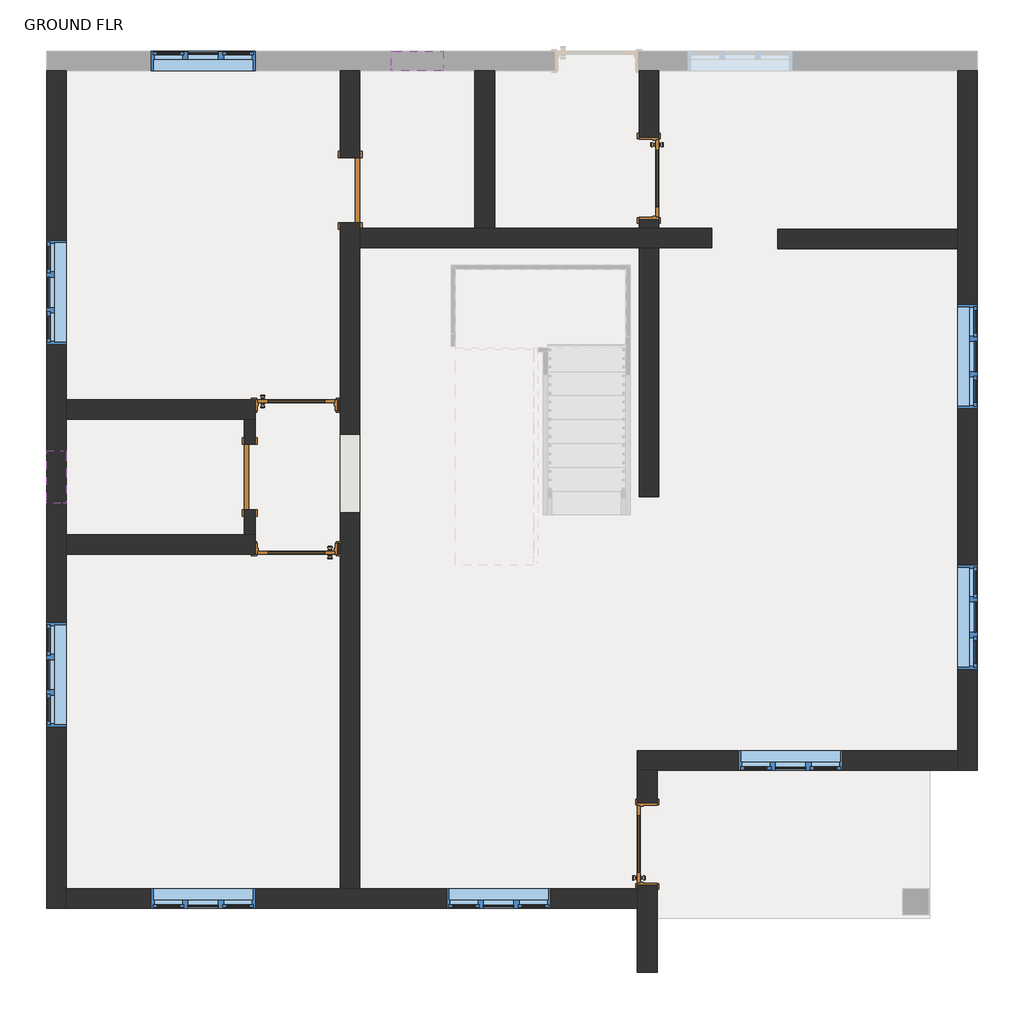
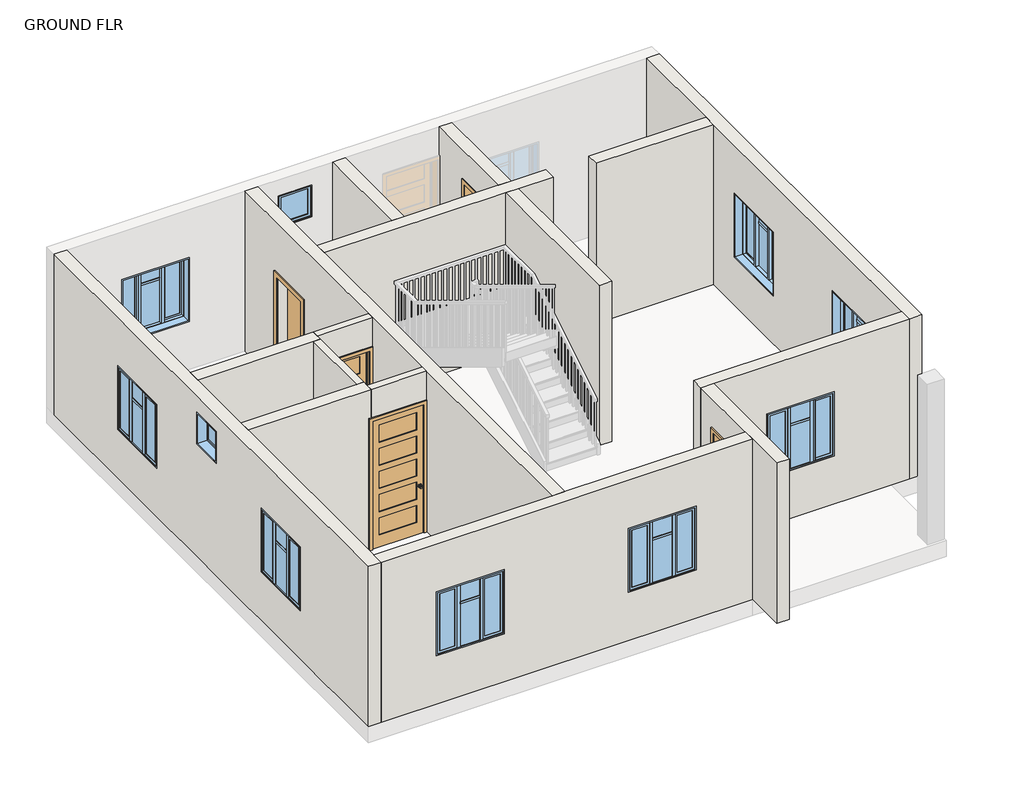
# One storey, part 1 of 3: 15 walls, 10 windows, 6 doors.
"""IFC4 building model written with IfcOpenShell, lengths in millimetres."""

from ifc_helpers import new_model, si_unit, point, frame, origin, place, context, project, spatial, polyline, ellipse_curve, trimmed, outline, extrude, faceted_brep, transform, mapped, element, save
from ifc_brep_helpers import plane_surface, extruded_surface, advanced_brep
from components import door_d793c26e, door_7b78131b, door_1fe7f57d, door_a1484949, window_80340324, window_casement_triple_middle_transom_window_4_x_4_1416bf83

model = new_model("IFC4")

# Units and contexts
model_context = context("Model", 3, world=origin())
ifc_project = project(units=[si_unit("LENGTHUNIT", "METRE", prefix="MILLI")], contexts=[model_context])

# Site, building, storey
site = spatial("IfcSite", under=ifc_project)
building = spatial("IfcBuilding", under=site)
storey = spatial("IfcBuildingStorey", under=building, Name="GROUND FLR", Elevation=609.6)

# Doors
placement = place(None, origin())
door_shape = door_d793c26e(model_context)
element("IfcDoor", 1, ObjectType="Door-Interior-Single-5_Panel_Vert-Wood : 36\" x 96\"", at=placement, inside=storey, context=model_context, shape_type="MappedRepresentation", body=[
    mapped(door_shape, transform((-5132.6956632, -7100.6948807, 609.6), x_axis=(0.0, 1.0, 0.0), y_axis=(-1.0, 0.0, 0.0), z_axis=(0.0, 0.0, 1.0))),
])
element("IfcDoor", 2, ObjectType="Door-Interior-Single-5_Panel_Vert-Wood : 36\" x 96\"", at=placement, inside=storey, context=model_context, shape_type="MappedRepresentation", body=[
    mapped(door_shape, transform((-5108.2681792, 684.4051193, 609.6), x_axis=(0.0, -1.0, 0.0), y_axis=(1.0, 0.0, 0.0), z_axis=(0.0, 0.0, 1.0))),
])
door_2_shape = door_7b78131b(model_context)
element("IfcDoor", 3, ObjectType="Door-Interior-Single-5_Panel_Vert-Wood : 36\" x 96\"", at=placement, inside=storey, context=model_context, shape_type="MappedRepresentation", body=[
    mapped(door_2_shape, transform((-9231.6206632, -3649.4698807, 609.6), x_axis=(-1.0, 0.0, 0.0), y_axis=(0.0, -1.0, 0.0), z_axis=(0.0, 0.0, 1.0))),
])
element("IfcDoor", 4, ObjectType="Door-Interior-Single-5_Panel_Vert-Wood : 36\" x 96\"", at=placement, inside=storey, context=model_context, shape_type="MappedRepresentation", body=[
    mapped(door_2_shape, transform((-9231.6206632, -1966.7198807, 609.6), x_axis=(1.0, 0.0, 0.0), y_axis=(0.0, 1.0, 0.0), z_axis=(0.0, 0.0, 1.0))),
])
door_3_shape = door_1fe7f57d(model_context)
element("IfcDoor", 5, ObjectType="Single-Flush : 30\" x 80\"", at=placement, inside=storey, context=model_context, shape_type="MappedRepresentation", body=[
    mapped(door_3_shape, transform((-9777.7206632, -2808.0948807, 609.6), x_axis=(0.0, 1.0, 0.0), y_axis=(-1.0, 0.0, 0.0), z_axis=(0.0, 0.0, 1.0))),
])
door_4_shape = door_a1484949(model_context)
element("IfcDoor", 6, ObjectType="Single-Flush : 30\" x 80\"", at=placement, inside=storey, context=model_context, shape_type="MappedRepresentation", body=[
    mapped(door_4_shape, transform((-8603.9431792, 544.7051193, 609.6), x_axis=(0.0, -1.0, 0.0), y_axis=(1.0, 0.0, 0.0), z_axis=(0.0, 0.0, 1.0))),
])

# Walls
element("IfcWall", 7, ObjectType="INTERIOR WALL 5\"", at=placement, inside=storey, context=model_context, shape_type="SweptSolid", body=[
    extrude(outline(polyline([(-2134.9948807, 609.6), (-2427.0948807, 609.6), (-2427.0948807, 2641.6), (-3189.0948807, 2641.6), (-3189.0948807, 609.6), (-3481.1948807, 609.6), (-3481.1948807, 3657.6), (-2134.9948807, 3657.6), (-2134.9948807, 609.6)])), frame((-9841.2206632, 0.0, 0.0), z_axis=(1.0, 0.0, 0.0), x_axis=(0.0, 1.0, 0.0)), (0.0, 0.0, 1.0), 127.0),
])
element("IfcWall", 8, ObjectType="INTERIOR WALL 5\"", at=placement, inside=storey, context=model_context, shape_type="SweptSolid", body=[
    extrude(outline(polyline([(3657.6, -8718.2431792), (3657.6, -9714.2206632), (3073.4, -9714.2206632), (3073.4, -8749.0206632), (609.6, -8749.0206632), (609.6, -8718.2431792), (3657.6, -8718.2431792)])), frame((0.0, -3709.7948807, 0.0), z_axis=(0.0, 1.0, 0.0), x_axis=(0.0, 0.0, 1.0)), (0.0, 0.0, 1.0), 127.0),
])
element("IfcWall", 9, ObjectType="INTERIOR WALL 5\"", at=placement, inside=storey, context=model_context, shape_type="SweptSolid", body=[
    extrude(outline(polyline([(3657.6, -8718.2431792), (3657.6, -9714.2206632), (3073.4, -9714.2206632), (3073.4, -8749.0206632), (609.6, -8749.0206632), (609.6, -8718.2431792), (3657.6, -8718.2431792)])), frame((0.0, -2033.3948807, 0.0), z_axis=(0.0, 1.0, 0.0), x_axis=(0.0, 0.0, 1.0)), (0.0, 0.0, 1.0), 127.0),
])
element("IfcWall", 10, ObjectType="WALL 9\"", at=placement, inside=storey, context=model_context, shape_type="Brep", body=[
    faceted_brep([(-12152.6206632, 1941.7051193, 609.6), (-12152.6206632, -7849.9948807, 609.6), (-12152.6206632, -7849.9948807, 3657.6), (-12152.6206632, 1941.7051193, 3657.6), (-12152.6206632, -39.4948807, 2743.2), (-12152.6206632, -1258.6948807, 2743.2), (-12152.6206632, -1258.6948807, 1524.0), (-12152.6206632, -39.4948807, 1524.0), (-12152.6206632, -4509.8948807, 2743.2), (-12152.6206632, -5729.0948807, 2743.2), (-12152.6206632, -5729.0948807, 1524.0), (-12152.6206632, -4509.8948807, 1524.0), (-12152.6206632, -3112.8948807, 3352.8), (-12152.6206632, -3112.8948807, 2743.2), (-12152.6206632, -2503.2948807, 2743.2), (-12152.6206632, -2503.2948807, 3352.8), (-11924.0206632, 1941.7051193, 609.6), (-11924.0206632, 1941.7051193, 3657.6), (-11924.0206632, -1906.3948807, 3657.6), (-11924.0206632, -2134.9948807, 3657.6), (-11924.0206632, -3481.1948807, 3657.6), (-11924.0206632, -3709.7948807, 3657.6), (-11924.0206632, -7621.3948807, 3657.6), (-11924.0206632, -7849.9948807, 3657.6), (-11924.0206632, -7849.9948807, 609.6), (-11924.0206632, -7621.3948807, 609.6), (-11924.0206632, -3709.7948807, 609.6), (-11924.0206632, -3481.1948807, 609.6), (-11924.0206632, -2134.9948807, 609.6), (-11924.0206632, -1906.3948807, 609.6), (-11924.0206632, -39.4948807, 2743.2), (-11924.0206632, -39.4948807, 1524.0), (-11924.0206632, -1258.6948807, 1524.0), (-11924.0206632, -1258.6948807, 2743.2), (-11924.0206632, -4509.8948807, 2743.2), (-11924.0206632, -4509.8948807, 1524.0), (-11924.0206632, -5729.0948807, 1524.0), (-11924.0206632, -5729.0948807, 2743.2), (-11924.0206632, -3112.8948807, 3352.8), (-11924.0206632, -2503.2948807, 3352.8), (-11924.0206632, -2503.2948807, 2743.2), (-11924.0206632, -3112.8948807, 2743.2)], [[[0, 1, 2, 3], [4, 5, 6, 7], [8, 9, 10, 11], [12, 13, 14, 15]], [[16, 17, 18, 19, 20, 21, 22, 23, 24, 25, 26, 27, 28, 29], [30, 31, 32, 33], [34, 35, 36, 37], [38, 39, 40, 41]], [[1, 0, 16, 29, 28, 27, 26, 25, 24]], [[3, 2, 23, 22, 21, 20, 19, 18, 17]], [[0, 3, 17, 16]], [[2, 1, 24, 23]], [[31, 30, 4, 7]], [[32, 31, 7, 6]], [[33, 32, 6, 5]], [[30, 33, 5, 4]], [[35, 34, 8, 11]], [[36, 35, 11, 10]], [[37, 36, 10, 9]], [[34, 37, 9, 8]], [[13, 12, 38, 41]], [[14, 13, 41, 40]], [[15, 14, 40, 39]], [[12, 15, 39, 38]]]),
])
element("IfcWall", 11, ObjectType="WALL 9\"", at=placement, inside=storey, context=model_context, shape_type="Brep", body=[
    faceted_brep([(-1497.3206632, 1941.7051193, 609.6), (-1497.3206632, 87.5051193, 609.6), (-1497.3206632, -141.0948807, 609.6), (-1497.3206632, -6008.4948807, 609.6), (-1497.3206632, -6237.0948807, 609.6), (-1497.3206632, -6237.0948807, 3657.6), (-1497.3206632, -6008.4948807, 3657.6), (-1497.3206632, -141.0948807, 3657.6), (-1497.3206632, 87.5051193, 3657.6), (-1497.3206632, 1941.7051193, 3657.6), (-1497.3206632, -5055.9948807, 2743.2), (-1497.3206632, -5055.9948807, 1524.0), (-1497.3206632, -3836.7948807, 1524.0), (-1497.3206632, -3836.7948807, 2743.2), (-1497.3206632, -2007.9948807, 2743.2), (-1497.3206632, -2007.9948807, 1524.0), (-1497.3206632, -788.7948807, 1524.0), (-1497.3206632, -788.7948807, 2743.2), (-1268.7206632, 1941.7051193, 609.6), (-1268.7206632, 1941.7051193, 3657.6), (-1268.7206632, -6237.0948807, 3657.6), (-1268.7206632, -6237.0948807, 609.6), (-1268.7206632, -5055.9948807, 2743.2), (-1268.7206632, -3836.7948807, 2743.2), (-1268.7206632, -3836.7948807, 1524.0), (-1268.7206632, -5055.9948807, 1524.0), (-1268.7206632, -2007.9948807, 2743.2), (-1268.7206632, -788.7948807, 2743.2), (-1268.7206632, -788.7948807, 1524.0), (-1268.7206632, -2007.9948807, 1524.0)], [[[0, 1, 2, 3, 4, 5, 6, 7, 8, 9], [10, 11, 12, 13], [14, 15, 16, 17]], [[18, 19, 20, 21], [22, 23, 24, 25], [26, 27, 28, 29]], [[4, 3, 2, 1, 0, 18, 21]], [[9, 8, 7, 6, 5, 20, 19]], [[0, 9, 19, 18]], [[5, 4, 21, 20]], [[11, 10, 22, 25]], [[12, 11, 25, 24]], [[13, 12, 24, 23]], [[10, 13, 23, 22]], [[15, 14, 26, 29]], [[16, 15, 29, 28]], [[17, 16, 28, 27]], [[14, 17, 27, 26]]]),
])
element("IfcWall", 12, ObjectType="WALL 9\"", at=placement, inside=storey, context=model_context, shape_type="SweptSolid", body=[
    extrude(outline(polyline([(-3605.5206632, 87.5051193), (-1497.3206632, 87.5051193), (-1497.3206632, -141.0948807), (-3605.5206632, -141.0948807), (-3605.5206632, 87.5051193)])), frame((0.0, 0.0, 609.6), z_axis=(0.0, 0.0, 1.0), x_axis=(1.0, 0.0, 0.0)), (0.0, 0.0, 1.0), 3048.0),
])
element("IfcWall", 13, ObjectType="WALL 9\"", at=placement, inside=storey, context=model_context, shape_type="Brep", body=[
    faceted_brep([(-11924.0206632, -7849.9948807, 609.6), (-5243.8206632, -7849.9948807, 609.6), (-5243.8206632, -7849.9948807, 3657.6), (-11924.0206632, -7849.9948807, 3657.6), (-10930.7319212, -7849.9948807, 2743.2), (-9711.5319212, -7849.9948807, 2743.2), (-9711.5319212, -7849.9948807, 1524.0), (-10930.7319212, -7849.9948807, 1524.0), (-7476.3319212, -7849.9948807, 2743.2), (-6257.1319212, -7849.9948807, 2743.2), (-6257.1319212, -7849.9948807, 1524.0), (-7476.3319212, -7849.9948807, 1524.0), (-11924.0206632, -7621.3948807, 609.6), (-11924.0206632, -7621.3948807, 3657.6), (-8718.2431792, -7621.3948807, 3657.6), (-8489.6431792, -7621.3948807, 3657.6), (-5243.8206632, -7621.3948807, 3657.6), (-5243.8206632, -7621.3948807, 609.6), (-8489.6431792, -7621.3948807, 609.6), (-8718.2431792, -7621.3948807, 609.6), (-10930.7319212, -7621.3948807, 2743.2), (-10930.7319212, -7621.3948807, 1524.0), (-9711.5319212, -7621.3948807, 1524.0), (-9711.5319212, -7621.3948807, 2743.2), (-7476.3319212, -7621.3948807, 2743.2), (-7476.3319212, -7621.3948807, 1524.0), (-6257.1319212, -7621.3948807, 1524.0), (-6257.1319212, -7621.3948807, 2743.2)], [[[0, 1, 2, 3], [4, 5, 6, 7], [8, 9, 10, 11]], [[12, 13, 14, 15, 16, 17, 18, 19], [20, 21, 22, 23], [24, 25, 26, 27]], [[1, 0, 12, 19, 18, 17]], [[3, 2, 16, 15, 14, 13]], [[0, 3, 13, 12]], [[2, 1, 17, 16]], [[21, 20, 4, 7]], [[22, 21, 7, 6]], [[23, 22, 6, 5]], [[20, 23, 5, 4]], [[25, 24, 8, 11]], [[26, 25, 11, 10]], [[27, 26, 10, 9]], [[24, 27, 9, 8]]]),
])
element("IfcWall", 14, ObjectType="WALL 9\"", at=placement, inside=storey, context=model_context, shape_type="Brep", body=[
    faceted_brep([(-5015.2206632, -6237.0948807, 3657.6), (-5015.2206632, -8599.2948807, 3657.6), (-5015.2206632, -8599.2948807, 609.6), (-5015.2206632, -7583.2948807, 609.6), (-5015.2206632, -7583.2948807, 3073.4), (-5015.2206632, -6618.0948807, 3073.4), (-5015.2206632, -6618.0948807, 609.6), (-5015.2206632, -6237.0948807, 609.6), (-5243.8206632, -8599.2948807, 3657.6), (-5243.8206632, -7849.9948807, 3657.6), (-5243.8206632, -7621.3948807, 3657.6), (-5243.8206632, -6237.0948807, 3657.6), (-5243.8206632, -6237.0948807, 609.6), (-5243.8206632, -6618.0948807, 609.6), (-5243.8206632, -6618.0948807, 3073.4), (-5243.8206632, -7583.2948807, 3073.4), (-5243.8206632, -7583.2948807, 609.6), (-5243.8206632, -7621.3948807, 609.6), (-5243.8206632, -7849.9948807, 609.6), (-5243.8206632, -8599.2948807, 609.6)], [[[0, 1, 2, 3, 4, 5, 6, 7]], [[8, 9, 10, 11, 12, 13, 14, 15, 16, 17, 18, 19]], [[2, 19, 18, 17, 16, 3]], [[12, 7, 6, 13]], [[1, 0, 11, 10, 9, 8]], [[2, 1, 8, 19]], [[0, 7, 12, 11]], [[5, 14, 13, 6]], [[14, 5, 4, 15]], [[15, 4, 3, 16]]]),
])
element("IfcWall", 15, ObjectType="WALL 9\"", at=placement, inside=storey, context=model_context, shape_type="AdvancedBrep", body=[
    advanced_brep(
    [(-8489.6431792, -7621.3948807, 609.6), (-8489.6431792, -128.3948807, 609.6), (-8489.6431792, 100.2051193, 609.6), (-8489.6431792, 163.7051193, 609.6), (-8489.6431792, 163.7051193, 2641.6), (-8489.6431792, 925.7051193, 2641.6), (-8489.6431792, 925.7051193, 609.6), (-8489.6431792, 1941.7051193, 609.6), (-8489.6431792, 1941.7051193, 3657.6), (-8489.6431792, 100.2051193, 3657.6), (-8489.6431792, -128.3948807, 3657.6), (-8489.6431792, -7621.3948807, 3657.6), (-8489.6431792, -3223.1355399, 2260.764257), (-8489.6431792, -2308.7355399, 2260.764257), (-8489.6431792, -2308.7355399, 635.164257), (-8489.6431792, -3223.1355399, 635.164257), (-8718.2431792, 163.7051193, 2641.6), (-8718.2431792, 163.7051193, 609.6), (-8718.2431792, -1906.3948807, 609.6), (-8718.2431792, -2033.3948807, 609.6), (-8718.2431792, -3582.7948807, 609.6), (-8718.2431792, -3709.7948807, 609.6), (-8718.2431792, -7621.3948807, 609.6), (-8718.2431792, -7621.3948807, 3657.6), (-8718.2431792, -3709.7948807, 3657.6), (-8718.2431792, -3582.7948807, 3657.6), (-8718.2431792, -2033.3948807, 3657.6), (-8718.2431792, -1906.3948807, 3657.6), (-8718.2431792, 1941.7051193, 3657.6), (-8718.2431792, 1941.7051193, 609.6), (-8718.2431792, 925.7051193, 609.6), (-8718.2431792, 925.7051193, 2641.6), (-8718.2431792, -3223.1355399, 2260.764257), (-8718.2431792, -3223.1355399, 635.164257), (-8718.2431792, -2308.7355399, 635.164257), (-8718.2431792, -2308.7355399, 2260.764257)],
    [
        (0, 1),
        (1, 2),
        (2, 3),
        (3, 4),
        (4, 5),
        (5, 6),
        (6, 7),
        (7, 8),
        (8, 9),
        (9, 10),
        (10, 11),
        (11, 0),
        (12, 13, ellipse_curve(frame((-8489.6431792, -2765.9355399, 2260.764257), z_axis=(-1.0, 0.0, 0.0), x_axis=(0.0, 1.0, 0.0)), 457.2, 431.8)),
        (13, 14),
        (14, 15),
        (15, 12),
        (16, 17),
        (17, 18),
        (18, 19),
        (19, 20),
        (20, 21),
        (21, 22),
        (22, 23),
        (23, 24),
        (24, 25),
        (25, 26),
        (26, 27),
        (27, 28),
        (28, 29),
        (29, 30),
        (30, 31),
        (31, 16),
        (32, 33),
        (33, 34),
        (34, 35),
        (35, 32, ellipse_curve(frame((-8718.2431792, -2765.9355399, 2260.764257), z_axis=(1.0, 0.0, 0.0), x_axis=(0.0, 1.0, 0.0)), 457.2, 431.8)),
        (11, 23),
        (22, 0),
        (7, 29),
        (28, 8),
        (6, 30),
        (17, 3),
        (15, 33),
        (32, 12),
        (35, 13),
        (34, 14),
        (16, 4),
        (31, 5),
    ],
    [
        plane_surface(frame((-8489.6431792, -7589.8597576, 609.6), z_axis=(1.0, 0.0, 0.0), x_axis=(0.0, 1.0, 0.0))),
        plane_surface(frame((-8718.2431792, -7589.8597576, 609.6), z_axis=(-1.0, 0.0, 0.0), x_axis=(0.0, -1.0, 0.0))),
        plane_surface(frame((-11924.0206632, -7621.3948807, 609.6), z_axis=(0.0, -1.0, 0.0), x_axis=(-1.0, 0.0, 0.0))),
        plane_surface(frame((-12018.5080337, 1941.7051193, 609.6), z_axis=(0.0, 1.0, 0.0), x_axis=(1.0, 0.0, 0.0))),
        plane_surface(frame((-8489.6431792, -7735.6948807, 609.6), z_axis=(0.0, 0.0, -1.0), x_axis=(-1.0, 0.0, 0.0))),
        plane_surface(frame((-8489.6431792, 2056.0051193, 3657.6), z_axis=(0.0, 0.0, 1.0), x_axis=(-1.0, 0.0, 0.0))),
        plane_surface(frame((-8489.6431792, -3223.1355399, 635.164257), z_axis=(0.0, 1.0, 0.0), x_axis=(-1.0, 0.0, 0.0))),
        extruded_surface(trimmed(ellipse_curve(frame((-8832.5431792, -2765.9355399, 2260.764257), z_axis=(-1.0, 0.0, 0.0), x_axis=(0.0, 1.0, 0.0)), 457.2, 431.8), [point((-8832.5431792, -3223.1355399, 2260.764257))], [point((-8832.5431792, -2308.7355399, 2260.764257))], True, "CARTESIAN"), (228.60000000000036, 0.0, 0.0), 228.60000000000036),
        plane_surface(frame((-8489.6431792, -2308.7355399, 2260.764257), z_axis=(0.0, -1.0, 0.0), x_axis=(-1.0, 0.0, 0.0))),
        plane_surface(frame((-8489.6431792, -2308.7355399, 635.164257), z_axis=(0.0, 0.0, 1.0), x_axis=(-1.0, 0.0, 0.0))),
        plane_surface(frame((-8489.6431792, 163.7051193, 609.6), z_axis=(0.0, 1.0, 0.0), x_axis=(-1.0, 0.0, 0.0))),
        plane_surface(frame((-8489.6431792, 163.7051193, 2641.6), z_axis=(0.0, 0.0, -1.0), x_axis=(-1.0, 0.0, 0.0))),
        plane_surface(frame((-8489.6431792, 925.7051193, 2641.6), z_axis=(0.0, -1.0, 0.0), x_axis=(-1.0, 0.0, 0.0))),
    ],
    [
        (0, [[1, 2, 3, 4, 5, 6, 7, 8, 9, 10, 11, 12], [13, 14, 15, 16]]),
        (1, [[17, 18, 19, 20, 21, 22, 23, 24, 25, 26, 27, 28, 29, 30, 31, 32], [33, 34, 35, 36]]),
        (2, [[-12, 37, -23, 38]]),
        (3, [[-8, 39, -29, 40]]),
        (4, [[-30, -39, -7, 41]]),
        (4, [[-22, -21, -20, -19, -18, 42, -3, -2, -1, -38]]),
        (5, [[-11, -10, -9, -40, -28, -27, -26, -25, -24, -37]]),
        (6, [[-16, 43, -33, 44]]),
        (7, [[-13, -44, -36, 45]]),
        (8, [[-14, -45, -35, 46]]),
        (9, [[-15, -46, -34, -43]]),
        (10, [[-4, -42, -17, 47]]),
        (11, [[-5, -47, -32, 48]]),
        (12, [[-6, -48, -31, -41]]),
    ],
),
])
element("IfcWall", 16, ObjectType="WALL 9\"", at=placement, inside=storey, context=model_context, shape_type="Brep", body=[
    faceted_brep([(-8489.6431792, -128.3948807, 609.6), (-5225.7431792, -128.3948807, 609.6), (-4997.1431792, -128.3948807, 609.6), (-4374.8431792, -128.3948807, 609.6), (-4374.8431792, -128.3948807, 3657.6), (-4997.1431792, -128.3948807, 3657.6), (-5225.7431792, -128.3948807, 3657.6), (-8489.6431792, -128.3948807, 3657.6), (-8489.6431792, 100.2051193, 609.6), (-8489.6431792, 100.2051193, 3657.6), (-7143.4431792, 100.2051193, 3657.6), (-6914.8431792, 100.2051193, 3657.6), (-5225.7431792, 100.2051193, 3657.6), (-4997.1431792, 100.2051193, 3657.6), (-4374.8431792, 100.2051193, 3657.6), (-4374.8431792, 100.2051193, 609.6), (-4997.1431792, 100.2051193, 609.6), (-5225.7431792, 100.2051193, 609.6), (-6914.8431792, 100.2051193, 609.6), (-7143.4431792, 100.2051193, 609.6)], [[[0, 1, 2, 3, 4, 5, 6, 7]], [[8, 9, 10, 11, 12, 13, 14, 15, 16, 17, 18, 19]], [[3, 2, 1, 0, 8, 19, 18, 17, 16, 15]], [[4, 3, 15, 14]], [[7, 6, 5, 4, 14, 13, 12, 11, 10, 9]], [[0, 7, 9, 8]]]),
])
element("IfcWall", 17, ObjectType="WALL 9\"", at=placement, inside=storey, context=model_context, shape_type="SweptSolid", body=[
    extrude(outline(polyline([(-7143.4431792, 100.2051193), (-7143.4431792, 1941.7051193), (-6914.8431792, 1941.7051193), (-6914.8431792, 100.2051193), (-7143.4431792, 100.2051193)])), frame((0.0, 0.0, 609.6), z_axis=(0.0, 0.0, 1.0), x_axis=(1.0, 0.0, 0.0)), (0.0, 0.0, 1.0), 3048.0),
])
element("IfcWall", 18, ObjectType="WALL 9\"", at=placement, inside=storey, context=model_context, shape_type="SweptSolid", body=[
    extrude(outline(polyline([(-4997.1431792, -3036.6948807), (-5225.7431792, -3036.6948807), (-5225.7431792, -128.3948807), (-4997.1431792, -128.3948807), (-4997.1431792, -3036.6948807)])), frame((0.0, 0.0, 609.6), z_axis=(0.0, 0.0, 1.0), x_axis=(1.0, 0.0, 0.0)), (0.0, 0.0, 1.0), 3048.0),
    extrude(outline(polyline([(1941.7051193, 3657.6), (1941.7051193, 609.6), (1167.0051193, 609.6), (1167.0051193, 3073.4), (201.8051193, 3073.4), (201.8051193, 609.6), (100.2051193, 609.6), (100.2051193, 3657.6), (1941.7051193, 3657.6)])), frame((-5225.7431792, 0.0, 0.0), z_axis=(1.0, 0.0, 0.0), x_axis=(0.0, 1.0, 0.0)), (0.0, 0.0, 1.0), 228.6),
])
element("IfcWall", 19, ObjectType="WALL 9\"", at=placement, inside=storey, context=model_context, shape_type="Brep", body=[
    faceted_brep([(-1497.3206632, -6008.4948807, 609.6), (-5243.8206632, -6008.4948807, 609.6), (-5243.8206632, -6008.4948807, 3657.6), (-1497.3206632, -6008.4948807, 3657.6), (-4062.7206632, -6008.4948807, 2743.2), (-4062.7206632, -6008.4948807, 1524.0), (-2843.5206632, -6008.4948807, 1524.0), (-2843.5206632, -6008.4948807, 2743.2), (-1497.3206632, -6237.0948807, 609.6), (-1497.3206632, -6237.0948807, 3657.6), (-5015.2206632, -6237.0948807, 3657.6), (-5243.8206632, -6237.0948807, 3657.6), (-5243.8206632, -6237.0948807, 609.6), (-5015.2206632, -6237.0948807, 609.6), (-4062.7206632, -6237.0948807, 2743.2), (-2843.5206632, -6237.0948807, 2743.2), (-2843.5206632, -6237.0948807, 1524.0), (-4062.7206632, -6237.0948807, 1524.0)], [[[0, 1, 2, 3], [4, 5, 6, 7]], [[8, 9, 10, 11, 12, 13], [14, 15, 16, 17]], [[1, 0, 8, 13, 12]], [[3, 2, 11, 10, 9]], [[0, 3, 9, 8]], [[2, 1, 12, 11]], [[5, 4, 14, 17]], [[6, 5, 17, 16]], [[7, 6, 16, 15]], [[4, 7, 15, 14]]]),
])
element("IfcWall", 20, ObjectType="WALL 9\"", at=placement, inside=storey, context=model_context, shape_type="Brep", body=[
    faceted_brep([(-11924.0206632, -2134.9948807, 609.6), (-9841.2206632, -2134.9948807, 609.6), (-9714.2206632, -2134.9948807, 609.6), (-9714.2206632, -2134.9948807, 3657.6), (-9841.2206632, -2134.9948807, 3657.6), (-11924.0206632, -2134.9948807, 3657.6), (-11924.0206632, -1906.3948807, 609.6), (-11924.0206632, -1906.3948807, 3657.6), (-9714.2206632, -1906.3948807, 3657.6), (-9714.2206632, -1906.3948807, 3073.4), (-9714.2206632, -1906.3948807, 609.6), (-9714.2206632, -2033.3948807, 3657.6)], [[[0, 1, 2, 3, 4, 5]], [[6, 7, 8, 9, 10]], [[2, 1, 0, 6, 10]], [[5, 4, 3, 11, 8, 7]], [[0, 5, 7, 6]], [[3, 2, 10, 9, 8, 11]]]),
])
element("IfcWall", 21, ObjectType="WALL 9\"", at=placement, inside=storey, context=model_context, shape_type="Brep", body=[
    faceted_brep([(-11924.0206632, -3709.7948807, 609.6), (-9714.2206632, -3709.7948807, 609.6), (-9714.2206632, -3709.7948807, 3073.4), (-9714.2206632, -3709.7948807, 3657.6), (-11924.0206632, -3709.7948807, 3657.6), (-11924.0206632, -3481.1948807, 609.6), (-11924.0206632, -3481.1948807, 3657.6), (-9841.2206632, -3481.1948807, 3657.6), (-9714.2206632, -3481.1948807, 3657.6), (-9714.2206632, -3481.1948807, 609.6), (-9841.2206632, -3481.1948807, 609.6), (-9714.2206632, -3582.7948807, 3657.6)], [[[0, 1, 2, 3, 4]], [[5, 6, 7, 8, 9, 10]], [[1, 0, 5, 10, 9]], [[4, 3, 11, 8, 7, 6]], [[0, 4, 6, 5]], [[3, 2, 1, 9, 8, 11]]]),
])

# Windows
window_shape = window_80340324(model_context)
element("IfcWindow", 22, ObjectType="Fixed : 24\" x 24\"", at=placement, inside=storey, context=model_context, shape_type="MappedRepresentation", body=[
    mapped(window_shape, transform((-7854.6431792, 2056.0051193, 1828.8), x_axis=(-1.0, 0.0, 0.0), y_axis=(0.0, -1.0, 0.0), z_axis=(0.0, 0.0, 1.0))),
])
element("IfcWindow", 23, ObjectType="Fixed : 24\" x 24\"", at=placement, inside=storey, context=model_context, shape_type="MappedRepresentation", body=[
    mapped(window_shape, transform((-12038.3206632, -2846.1948807, 1828.8), x_axis=(0.0, -1.0, 0.0), y_axis=(1.0, 0.0, 0.0), z_axis=(0.0, 0.0, 1.0))),
])
window_casement_triple_middle_transom_window_4_x_4_shape = window_casement_triple_middle_transom_window_4_x_4_1416bf83(model_context)
element("IfcWindow", 24, ObjectType="Window-Casement-Triple-Middle-Transom : WINDOW 4' X 4'", at=placement, inside=storey, context=model_context, shape_type="MappedRepresentation", body=[
    mapped(window_casement_triple_middle_transom_window_4_x_4_shape, transform((-10321.1319212, 2056.0051193, 609.6), x_axis=(1.0, 0.0, 0.0), y_axis=(0.0, 1.0, 0.0), z_axis=(0.0, 0.0, 1.0))),
])
element("IfcWindow", 25, ObjectType="Window-Casement-Triple-Middle-Transom : WINDOW 4' X 4'", at=placement, inside=storey, context=model_context, shape_type="MappedRepresentation", body=[
    mapped(window_casement_triple_middle_transom_window_4_x_4_shape, transform((-12038.3206632, -649.0948807, 609.6), x_axis=(0.0, 1.0, 0.0), y_axis=(-1.0, 0.0, 0.0), z_axis=(0.0, 0.0, 1.0))),
])
element("IfcWindow", 26, ObjectType="Window-Casement-Triple-Middle-Transom : WINDOW 4' X 4'", at=placement, inside=storey, context=model_context, shape_type="MappedRepresentation", body=[
    mapped(window_casement_triple_middle_transom_window_4_x_4_shape, transform((-12038.3206632, -5119.4948807, 609.6), x_axis=(0.0, 1.0, 0.0), y_axis=(-1.0, 0.0, 0.0), z_axis=(0.0, 0.0, 1.0))),
])
element("IfcWindow", 27, ObjectType="Window-Casement-Triple-Middle-Transom : WINDOW 4' X 4'", at=placement, inside=storey, context=model_context, shape_type="MappedRepresentation", body=[
    mapped(window_casement_triple_middle_transom_window_4_x_4_shape, transform((-10321.1319212, -7735.6948807, 609.6), x_axis=(-1.0, 0.0, 0.0), y_axis=(0.0, -1.0, 0.0), z_axis=(0.0, 0.0, 1.0))),
])
element("IfcWindow", 28, ObjectType="Window-Casement-Triple-Middle-Transom : WINDOW 4' X 4'", at=placement, inside=storey, context=model_context, shape_type="MappedRepresentation", body=[
    mapped(window_casement_triple_middle_transom_window_4_x_4_shape, transform((-6866.7319212, -7735.6948807, 609.6), x_axis=(-1.0, 0.0, 0.0), y_axis=(0.0, -1.0, 0.0), z_axis=(0.0, 0.0, 1.0))),
])
element("IfcWindow", 29, ObjectType="Window-Casement-Triple-Middle-Transom : WINDOW 4' X 4'", at=placement, inside=storey, context=model_context, shape_type="MappedRepresentation", body=[
    mapped(window_casement_triple_middle_transom_window_4_x_4_shape, transform((-3453.1206632, -6122.7948807, 609.6), x_axis=(-1.0, 0.0, 0.0), y_axis=(0.0, -1.0, 0.0), z_axis=(0.0, 0.0, 1.0))),
])
element("IfcWindow", 30, ObjectType="Window-Casement-Triple-Middle-Transom : WINDOW 4' X 4'", at=placement, inside=storey, context=model_context, shape_type="MappedRepresentation", body=[
    mapped(window_casement_triple_middle_transom_window_4_x_4_shape, transform((-1383.0206632, -4446.3948807, 609.6), x_axis=(0.0, -1.0, 0.0), y_axis=(1.0, 0.0, 0.0), z_axis=(0.0, 0.0, 1.0))),
])
element("IfcWindow", 31, ObjectType="Window-Casement-Triple-Middle-Transom : WINDOW 4' X 4'", at=placement, inside=storey, context=model_context, shape_type="MappedRepresentation", body=[
    mapped(window_casement_triple_middle_transom_window_4_x_4_shape, transform((-1383.0206632, -1398.3948807, 609.6), x_axis=(0.0, -1.0, 0.0), y_axis=(1.0, 0.0, 0.0), z_axis=(0.0, 0.0, 1.0))),
])

save(model, "model.ifc")

# Revit data of these elements
# Type "Door-Interior-Single-5_Panel_Vert-Wood : 36\" x 96\""
#   Type Mark = "8"
#   Assembly Code = "C1020300"
#   Analytic Construction = "Wooden"
#   Top Rail = 0' - 4 11/16"
#   Thickness = 0' - 1 3/8"
#   Thermal Resistance (R) = 2.5876 (h·ft²·°F)/BTU
#   Swing Angle [instance default] = 90.00°
#   Stiles = 0' - 4 3/4"
#   Rough Width = 3' - 2"
#   Rough Height = 8' - 1"
#   Intermediate Rail = 0' - 4 1/2"
#   Height = 8' - 0"
#   Width = 3' - 0"
#   Heat Transfer Coefficient (U) = 0.3865 BTU/(h·ft²·°F)
#   Bottom Rail = 0' - 9 1/8"
#   Trim Material = Cherry
#   Panel Material = Cherry
#   Frame Material = Cherry
#   Door Handle Material = Aluminum
#   Visual Light Transmittance = 0
#   Solar Heat Gain Coefficient = 0
#   Wall Closure = (empty or 0)
#   Function = (empty or 0)
# Type "Single-Flush : 30\" x 80\""
#   Type Mark = "5"
#   Construction Type Id = "MDOOR"
#   Assembly Code = "C1020"
#   Analytic Construction = "Metal"
#   Thickness = 0' - 2"
#   Heat Transfer Coefficient (U) = 0.651978 BTU/(h·ft²·°F)
#   Height = 6' - 8"
#   Trim Projection Ext = 0' - 1"
#   Trim Projection Int = 0' - 1"
#   Trim Width = 0' - 3"
#   Width = 2' - 6"
#   Define Thermal Properties by = 1
#   Define Thermal Properties by = 1
#   Door Material = Door - Panel
#   Frame Material = Door - Frame
#   Visual Light Transmittance = 0
#   Solar Heat Gain Coefficient = 0
#   Function = (empty or 0)
#   Wall Closure = (empty or 0)
# Type "INTERIOR WALL 5\""
#   Assembly Code = "B2010"
#   Layers, outside or top first: 0' - 5" "SOFT COOL PAINT" (function 1)
# Type "WALL 9\""
#   Assembly Code = "B2010"
#   Layers, outside or top first: 0' - 9" "SOFT COOL PAINT" (function 1)
# Type "Fixed : 24\" x 24\""
#   Type Mark = "3"
#   Construction Type Id = "GSP4R"
#   Assembly Code = "B2020100"
#   Analytic Construction = "1/8 in Pilkington single glazing"
#   Visual Light Transmittance = 0.9
#   Solar Heat Gain Coefficient = 0.78
#   Heat Transfer Coefficient (U) = 0.6496 BTU/(h·ft²·°F)
#   Height = 2' - 0"
#   Default Sill Height = 3' - 0"
#   Width = 2' - 0"
#   Window Inset = 0' - 0 3/4"
#   Define Thermal Properties by = 1
#   Define Thermal Properties by = 1
#   Glass Pane Material = Glass
#   Sash Material = Sash
#   Wall Closure = (empty or 0)
# Type "Window-Casement-Triple-Middle-Transom : WINDOW 4' X 4'"
#   Type Mark = "21"
#   Fire Rating = "0.5h"
#   Assembly Code = "B2020100"
#   Analytic Construction = "Double glazing - domestic"
#   Window Width = 1' - 4"
#   Window Inset [instance default] = 0' - 0 5/8"
#   Wall Thickness [instance default] = 0' - 6"
#   Visual Light Transmittance = 0.81
#   Transom Height Ratio = 0.3
#   Thermal Resistance (R) = 1.8146 (h·ft²·°F)/BTU
#   Solar Heat Gain Coefficient = 0.76
#   Rough Width = 4' - 0 1/2"
#   Rough Height = 4' - 0 1/2"
#   Heat Transfer Coefficient (U) = 0.5511 BTU/(h·ft²·°F)
#   Height = 4' - 0"
#   Transom Height = 1' - 2.4"
#   Frame Gap 3 [instance default] = 0' - 1 83/128"
#   Frame Gap 2 [instance default] = 0' - 0 5/8"
#   Frame Gap 1 = 0' - 1 51/128"
#   Default Sill Height = 3' - 0"
#   Width = 4' - 0"
#   Frame Material = WOOD MATERIAL
#   Glass Panel Material = GLASS MATERIAL
#   Wall Closure = (empty or 0)
# Elements 1, 2, 3, 4 (IfcDoor, "Door-Interior-Single-5_Panel_Vert-Wood : 36\" x 96\"")
#   Swing Angle = 90.00°
#   Phase Created = New Construction
#   Materials on its faces: "Cherry", "Aluminum"
# Elements 5, 6 (IfcDoor, "Single-Flush : 30\" x 80\"")
#   Phase Created = New Construction
#   Materials on its faces: "Door - Frame", "Door - Panel"
# Elements 7, 8, 9 (IfcWall, "INTERIOR WALL 5\"")
#   Top Offset = 0' - 0"
#   Base Offset = 0' - 0"
#   wall height = 10' - 0"
#   Phase Created = New Construction
#   Base Constraint = GROUND FLR
#   Top Constraint = FIRST FLR
#   Materials on its faces: "SOFT COOL PAINT"
# Elements 10, 11, 12, 13, 14, 15, 16, 17, 18, 19, 20, 21 (IfcWall, "WALL 9\"")
#   Top Offset = 0' - 0"
#   Base Offset = 0' - 0"
#   wall height = 10' - 0"
#   Phase Created = New Construction
#   Base Constraint = GROUND FLR
#   Top Constraint = FIRST FLR
#   Materials on its faces: "SOFT COOL PAINT"
# Element 22 (IfcWindow, "Fixed : 24\" x 24\"")
#   Mark = "10"
#   Phase Created = New Construction
#   Materials on its faces: "Sash", "Glass"
# Element 23 (IfcWindow, "Fixed : 24\" x 24\"")
#   Mark = "11"
#   Phase Created = New Construction
#   Materials on its faces: "Sash", "Glass"
# Element 24 (IfcWindow, "Window-Casement-Triple-Middle-Transom : WINDOW 4' X 4'")
#   Mark = "1"
#   Window Inset = 0' - 0 5/8"
#   Frame Gap 3 = 0' - 1 83/128"
#   Frame Gap 2 = 0' - 0 5/8"
#   Phase Created = New Construction
#   Materials on its faces: "WOOD MATERIAL", "GLASS MATERIAL"
# Element 25 (IfcWindow, "Window-Casement-Triple-Middle-Transom : WINDOW 4' X 4'")
#   Mark = "2"
#   Window Inset = 0' - 0 5/8"
#   Frame Gap 3 = 0' - 1 83/128"
#   Frame Gap 2 = 0' - 0 5/8"
#   Phase Created = New Construction
#   Materials on its faces: "WOOD MATERIAL", "GLASS MATERIAL"
# Element 26 (IfcWindow, "Window-Casement-Triple-Middle-Transom : WINDOW 4' X 4'")
#   Mark = "3"
#   Window Inset = 0' - 0 5/8"
#   Frame Gap 3 = 0' - 1 83/128"
#   Frame Gap 2 = 0' - 0 5/8"
#   Phase Created = New Construction
#   Materials on its faces: "WOOD MATERIAL", "GLASS MATERIAL"
# Element 27 (IfcWindow, "Window-Casement-Triple-Middle-Transom : WINDOW 4' X 4'")
#   Mark = "4"
#   Window Inset = 0' - 0 5/8"
#   Frame Gap 3 = 0' - 1 83/128"
#   Frame Gap 2 = 0' - 0 5/8"
#   Phase Created = New Construction
#   Materials on its faces: "WOOD MATERIAL", "GLASS MATERIAL"
# Element 28 (IfcWindow, "Window-Casement-Triple-Middle-Transom : WINDOW 4' X 4'")
#   Mark = "5"
#   Window Inset = 0' - 0 5/8"
#   Frame Gap 3 = 0' - 1 83/128"
#   Frame Gap 2 = 0' - 0 5/8"
#   Phase Created = New Construction
#   Materials on its faces: "WOOD MATERIAL", "GLASS MATERIAL"
# Element 29 (IfcWindow, "Window-Casement-Triple-Middle-Transom : WINDOW 4' X 4'")
#   Mark = "6"
#   Window Inset = 0' - 0 5/8"
#   Frame Gap 3 = 0' - 1 83/128"
#   Frame Gap 2 = 0' - 0 5/8"
#   Phase Created = New Construction
#   Materials on its faces: "WOOD MATERIAL", "GLASS MATERIAL"
# Element 30 (IfcWindow, "Window-Casement-Triple-Middle-Transom : WINDOW 4' X 4'")
#   Mark = "7"
#   Window Inset = 0' - 0 5/8"
#   Frame Gap 3 = 0' - 1 83/128"
#   Frame Gap 2 = 0' - 0 5/8"
#   Phase Created = New Construction
#   Materials on its faces: "WOOD MATERIAL", "GLASS MATERIAL"
# Element 31 (IfcWindow, "Window-Casement-Triple-Middle-Transom : WINDOW 4' X 4'")
#   Mark = "8"
#   Window Inset = 0' - 0 5/8"
#   Frame Gap 3 = 0' - 1 83/128"
#   Frame Gap 2 = 0' - 0 5/8"
#   Phase Created = New Construction
#   Materials on its faces: "WOOD MATERIAL", "GLASS MATERIAL"
# Materials
#   "Cherry": class "Wood", colour RGB 226 177 128, transparency 0, Description = "Prunus Serotina", Cost = 0
#   "Aluminum": class "Metal", colour RGB 247 247 247, transparency 0, Description = "Aluminum 6061", Cost = 0
#   "Door - Panel": class "Wood", colour RGB 210 159 95, transparency 0, Cost = 0
#   "Door - Frame": colour RGB 118 70 51, transparency 0, Cost = 0
#   "SOFT COOL PAINT": class "Generic", colour RGB 120 120 120, transparency 0, Cost = 0
#   "Glass": class "Glass", colour RGB 0 128 192, transparency 0.75, Description = "Soda Lime Glass", Cost = 0
#   "Sash": class "Wood", colour RGB 224 178 126, transparency 0, Cost = 0
#   "WOOD MATERIAL": class "Generic", colour RGB 120 120 120, transparency 0, Cost = 0
#   "GLASS MATERIAL": class "Generic", colour RGB 120 120 120, transparency 0, Cost = 0
# Room at (-7816.543, 1020.955) mm, phase "New Construction", upper level "GROUND FLR", upper offset 10' - 0", lower offset 0' - 0"
#   Number = "1"
#   Name = "TOILET"
# Room at (-6070.293, 1020.955) mm, phase "New Construction", upper level "GROUND FLR", upper offset 10' - 0", lower offset 0' - 0"
#   Number = "2"
#   Name = "FOYER"
# Room at (-10908.021, -2808.095) mm, phase "New Construction", upper level "GROUND FLR", upper offset 10' - 0", lower offset 0' - 0"
#   Number = "3"
#   Name = "TOILET"
# Room at (-10321.132, -5665.595) mm, phase "New Construction", upper level "GROUND FLR", upper offset 10' - 0", lower offset 0' - 0"
#   Number = "4"
#   Name = "BED ROOM"
# Room at (-6710.671, -2839.845) mm, phase "New Construction", upper level "GROUND FLR", upper offset 10' - 0", lower offset 0' - 0"
#   Number = "5"
#   Name = "DINING AND KITCHEN AREA"
# Room at (-9190.832, -2808.095) mm, phase "New Construction", upper level "GROUND FLR", upper offset 10' - 0", lower offset 0' - 0"
#   Number = "6"
#   Name = "Room"
# Room at (-10196.45, 167.481) mm, phase "New Construction", upper level "GROUND FLR", upper offset 10' - 0", lower offset 0' - 0"
#   Number = "7"
#   Name = "BED ROOM"
